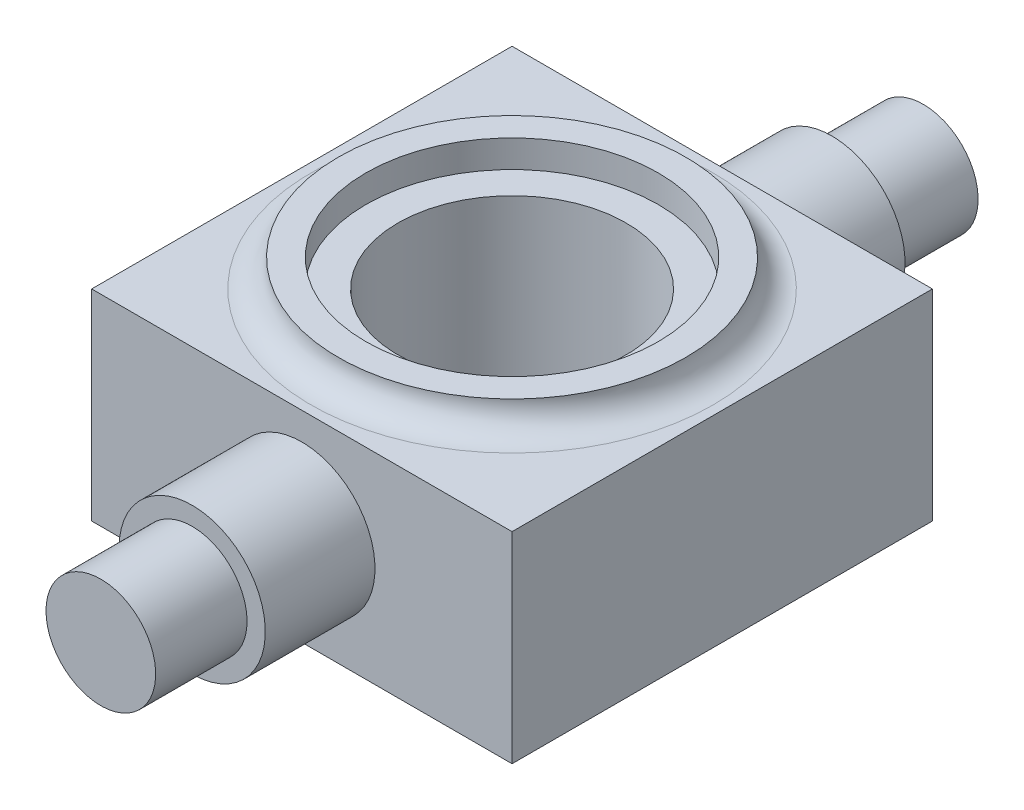
ISO-10303-21;
HEADER;
FILE_DESCRIPTION(('STEP AP214'),'2;1');
FILE_NAME('part.step','',(''),(''),'','','');
FILE_SCHEMA(('AUTOMOTIVE_DESIGN { 1 0 10303 214 1 1 1 1 }'));
ENDSEC;
DATA;
#1=APPLICATION_CONTEXT('core data for automotive mechanical design processes');
#2=APPLICATION_PROTOCOL_DEFINITION('international standard','automotive_design',2000,#1);
#3=PRODUCT_CONTEXT('',#1,'mechanical');
#4=PRODUCT('Part','Part','',(#3));
#5=PRODUCT_RELATED_PRODUCT_CATEGORY('part','',(#4));
#6=PRODUCT_DEFINITION_FORMATION('','',#4);
#7=PRODUCT_DEFINITION_CONTEXT('part definition',#1,'design');
#8=PRODUCT_DEFINITION('design','',#6,#7);
#9=PRODUCT_DEFINITION_SHAPE('','',#8);
#10=(LENGTH_UNIT() NAMED_UNIT(*) SI_UNIT(.MILLI.,.METRE.));
#11=(NAMED_UNIT(*) PLANE_ANGLE_UNIT() SI_UNIT($,.RADIAN.));
#12=(NAMED_UNIT(*) SI_UNIT($,.STERADIAN.) SOLID_ANGLE_UNIT());
#13=UNCERTAINTY_MEASURE_WITH_UNIT(LENGTH_MEASURE(1.E-05),#10,'distance_accuracy_value','');
#14=(GEOMETRIC_REPRESENTATION_CONTEXT(3) GLOBAL_UNCERTAINTY_ASSIGNED_CONTEXT((#13)) GLOBAL_UNIT_ASSIGNED_CONTEXT((#10,
#11,#12)) REPRESENTATION_CONTEXT('',''));
#15=CARTESIAN_POINT('',(0.,0.,0.));
#16=DIRECTION('',(0.,0.,1.));
#17=DIRECTION('',(1.,0.,0.));
#18=AXIS2_PLACEMENT_3D('',#15,#16,#17);
#19=CARTESIAN_POINT('',(-23.,-11.,23.));
#20=DIRECTION('',(1.,0.,0.));
#21=DIRECTION('',(0.,0.,-1.));
#22=AXIS2_PLACEMENT_3D('',#19,#20,#21);
#23=PLANE('',#22);
#24=DIRECTION('',(0.,-1.,0.));
#25=VECTOR('',#24,1.);
#26=CARTESIAN_POINT('',(-23.,-11.,-23.));
#27=LINE('',#26,#25);
#28=CARTESIAN_POINT('',(-23.,11.,-23.));
#29=VERTEX_POINT('',#28);
#30=CARTESIAN_POINT('',(-23.,-11.,-23.));
#31=VERTEX_POINT('',#30);
#32=EDGE_CURVE('E113',#29,#31,#27,.T.);
#33=ORIENTED_EDGE('',*,*,#32,.T.);
#34=DIRECTION('',(0.,0.,-1.));
#35=VECTOR('',#34,1.);
#36=CARTESIAN_POINT('',(-23.,-11.,23.));
#37=LINE('',#36,#35);
#38=CARTESIAN_POINT('',(-23.,-11.,23.));
#39=VERTEX_POINT('',#38);
#40=EDGE_CURVE('E104',#39,#31,#37,.T.);
#41=ORIENTED_EDGE('',*,*,#40,.F.);
#42=DIRECTION('',(0.,-1.,0.));
#43=VECTOR('',#42,1.);
#44=CARTESIAN_POINT('',(-23.,-11.,23.));
#45=LINE('',#44,#43);
#46=CARTESIAN_POINT('',(-23.,11.,23.));
#47=VERTEX_POINT('',#46);
#48=EDGE_CURVE('E96',#47,#39,#45,.T.);
#49=ORIENTED_EDGE('',*,*,#48,.F.);
#50=DIRECTION('',(0.,0.,-1.));
#51=VECTOR('',#50,1.);
#52=CARTESIAN_POINT('',(-23.,11.,23.));
#53=LINE('',#52,#51);
#54=EDGE_CURVE('E107',#47,#29,#53,.T.);
#55=ORIENTED_EDGE('',*,*,#54,.T.);
#56=EDGE_LOOP('',(#33,#41,#49,#55));
#57=FACE_BOUND('',#56,.T.);
#58=ADVANCED_FACE('F44',(#57),#23,.F.);
#59=CARTESIAN_POINT('',(23.,-11.,23.));
#60=DIRECTION('',(0.,1.,0.));
#61=DIRECTION('',(-1.,0.,0.));
#62=AXIS2_PLACEMENT_3D('',#59,#60,#61);
#63=PLANE('',#62);
#64=CARTESIAN_POINT('',(0.,-11.,0.));
#65=DIRECTION('',(0.,1.,0.));
#66=DIRECTION('',(-1.,0.,0.));
#67=AXIS2_PLACEMENT_3D('',#64,#65,#66);
#68=CIRCLE('',#67,22.);
#69=CARTESIAN_POINT('',(-22.,-11.,0.));
#70=VERTEX_POINT('',#69);
#71=EDGE_CURVE('E11',#70,#70,#68,.T.);
#72=ORIENTED_EDGE('',*,*,#71,.T.);
#73=EDGE_LOOP('',(#72));
#74=FACE_BOUND('',#73,.T.);
#75=DIRECTION('',(1.,0.,0.));
#76=VECTOR('',#75,1.);
#77=CARTESIAN_POINT('',(23.,-11.,-23.));
#78=LINE('',#77,#76);
#79=CARTESIAN_POINT('',(23.,-11.,-23.));
#80=VERTEX_POINT('',#79);
#81=EDGE_CURVE('E101',#31,#80,#78,.T.);
#82=ORIENTED_EDGE('',*,*,#81,.T.);
#83=DIRECTION('',(0.,0.,-1.));
#84=VECTOR('',#83,1.);
#85=CARTESIAN_POINT('',(23.,-11.,23.));
#86=LINE('',#85,#84);
#87=CARTESIAN_POINT('',(23.,-11.,23.));
#88=VERTEX_POINT('',#87);
#89=EDGE_CURVE('E103',#88,#80,#86,.T.);
#90=ORIENTED_EDGE('',*,*,#89,.F.);
#91=DIRECTION('',(1.,0.,0.));
#92=VECTOR('',#91,1.);
#93=CARTESIAN_POINT('',(23.,-11.,23.));
#94=LINE('',#93,#92);
#95=EDGE_CURVE('E95',#39,#88,#94,.T.);
#96=ORIENTED_EDGE('',*,*,#95,.F.);
#97=ORIENTED_EDGE('',*,*,#40,.T.);
#98=EDGE_LOOP('',(#82,#90,#96,#97));
#99=FACE_BOUND('',#98,.T.);
#100=ADVANCED_FACE('F105',(#74,#99),#63,.F.);
#101=CARTESIAN_POINT('',(23.,-11.,23.));
#102=DIRECTION('',(-1.,0.,0.));
#103=DIRECTION('',(0.,0.,1.));
#104=AXIS2_PLACEMENT_3D('',#101,#102,#103);
#105=PLANE('',#104);
#106=DIRECTION('',(0.,1.,0.));
#107=VECTOR('',#106,1.);
#108=CARTESIAN_POINT('',(23.,-11.,-23.));
#109=LINE('',#108,#107);
#110=CARTESIAN_POINT('',(23.,11.,-23.));
#111=VERTEX_POINT('',#110);
#112=EDGE_CURVE('E79',#80,#111,#109,.T.);
#113=ORIENTED_EDGE('',*,*,#112,.T.);
#114=DIRECTION('',(0.,0.,-1.));
#115=VECTOR('',#114,1.);
#116=CARTESIAN_POINT('',(23.,11.,23.));
#117=LINE('',#116,#115);
#118=CARTESIAN_POINT('',(23.,11.,23.));
#119=VERTEX_POINT('',#118);
#120=EDGE_CURVE('E102',#119,#111,#117,.T.);
#121=ORIENTED_EDGE('',*,*,#120,.F.);
#122=DIRECTION('',(0.,1.,0.));
#123=VECTOR('',#122,1.);
#124=CARTESIAN_POINT('',(23.,-11.,23.));
#125=LINE('',#124,#123);
#126=EDGE_CURVE('E98',#88,#119,#125,.T.);
#127=ORIENTED_EDGE('',*,*,#126,.F.);
#128=ORIENTED_EDGE('',*,*,#89,.T.);
#129=EDGE_LOOP('',(#113,#121,#127,#128));
#130=FACE_BOUND('',#129,.T.);
#131=ADVANCED_FACE('F110',(#130),#105,.F.);
#132=CARTESIAN_POINT('',(23.,11.,23.));
#133=DIRECTION('',(0.,-1.,0.));
#134=DIRECTION('',(1.,0.,0.));
#135=AXIS2_PLACEMENT_3D('',#132,#133,#134);
#136=PLANE('',#135);
#137=CARTESIAN_POINT('',(0.,11.,0.));
#138=DIRECTION('',(0.,-1.,0.));
#139=DIRECTION('',(1.,0.,0.));
#140=AXIS2_PLACEMENT_3D('',#137,#138,#139);
#141=CIRCLE('',#140,22.);
#142=CARTESIAN_POINT('',(22.,11.,0.));
#143=VERTEX_POINT('',#142);
#144=EDGE_CURVE('E53',#143,#143,#141,.T.);
#145=ORIENTED_EDGE('',*,*,#144,.T.);
#146=EDGE_LOOP('',(#145));
#147=FACE_BOUND('',#146,.T.);
#148=DIRECTION('',(-1.,0.,0.));
#149=VECTOR('',#148,1.);
#150=CARTESIAN_POINT('',(23.,11.,-23.));
#151=LINE('',#150,#149);
#152=EDGE_CURVE('E81',#111,#29,#151,.T.);
#153=ORIENTED_EDGE('',*,*,#152,.T.);
#154=ORIENTED_EDGE('',*,*,#54,.F.);
#155=DIRECTION('',(-1.,0.,0.));
#156=VECTOR('',#155,1.);
#157=CARTESIAN_POINT('',(23.,11.,23.));
#158=LINE('',#157,#156);
#159=EDGE_CURVE('E64',#119,#47,#158,.T.);
#160=ORIENTED_EDGE('',*,*,#159,.F.);
#161=ORIENTED_EDGE('',*,*,#120,.T.);
#162=EDGE_LOOP('',(#153,#154,#160,#161));
#163=FACE_BOUND('',#162,.T.);
#164=ADVANCED_FACE('F227',(#147,#163),#136,.F.);
#165=CARTESIAN_POINT('',(0.,0.,23.));
#166=DIRECTION('',(0.,0.,1.));
#167=DIRECTION('',(1.,0.,0.));
#168=AXIS2_PLACEMENT_3D('',#165,#166,#167);
#169=PLANE('',#168);
#170=CARTESIAN_POINT('',(0.,0.,23.));
#171=DIRECTION('',(0.,0.,-1.));
#172=DIRECTION('',(-1.,0.,0.));
#173=AXIS2_PLACEMENT_3D('',#170,#171,#172);
#174=CIRCLE('',#173,8.);
#175=CARTESIAN_POINT('',(-8.,0.,23.));
#176=VERTEX_POINT('',#175);
#177=EDGE_CURVE('E150',#176,#176,#174,.T.);
#178=ORIENTED_EDGE('',*,*,#177,.T.);
#179=EDGE_LOOP('',(#178));
#180=FACE_BOUND('',#179,.T.);
#181=ORIENTED_EDGE('',*,*,#48,.T.);
#182=ORIENTED_EDGE('',*,*,#95,.T.);
#183=ORIENTED_EDGE('',*,*,#126,.T.);
#184=ORIENTED_EDGE('',*,*,#159,.T.);
#185=EDGE_LOOP('',(#181,#182,#183,#184));
#186=FACE_BOUND('',#185,.T.);
#187=ADVANCED_FACE('F93',(#180,#186),#169,.T.);
#188=CARTESIAN_POINT('',(0.,0.,-23.));
#189=DIRECTION('',(0.,0.,1.));
#190=DIRECTION('',(1.,0.,0.));
#191=AXIS2_PLACEMENT_3D('',#188,#189,#190);
#192=PLANE('',#191);
#193=CARTESIAN_POINT('',(0.,0.,-23.));
#194=DIRECTION('',(0.,0.,-1.));
#195=DIRECTION('',(-1.,0.,0.));
#196=AXIS2_PLACEMENT_3D('',#193,#194,#195);
#197=CIRCLE('',#196,8.);
#198=CARTESIAN_POINT('',(-8.,0.,-23.));
#199=VERTEX_POINT('',#198);
#200=EDGE_CURVE('E124',#199,#199,#197,.T.);
#201=ORIENTED_EDGE('',*,*,#200,.F.);
#202=EDGE_LOOP('',(#201));
#203=FACE_BOUND('',#202,.T.);
#204=ORIENTED_EDGE('',*,*,#32,.F.);
#205=ORIENTED_EDGE('',*,*,#152,.F.);
#206=ORIENTED_EDGE('',*,*,#112,.F.);
#207=ORIENTED_EDGE('',*,*,#81,.F.);
#208=EDGE_LOOP('',(#204,#205,#206,#207));
#209=FACE_BOUND('',#208,.T.);
#210=ADVANCED_FACE('F230',(#203,#209),#192,.F.);
#211=CARTESIAN_POINT('',(0.,0.,-35.));
#212=DIRECTION('',(0.,0.,1.));
#213=DIRECTION('',(1.,0.,0.));
#214=AXIS2_PLACEMENT_3D('',#211,#212,#213);
#215=CYLINDRICAL_SURFACE('',#214,8.);
#216=CARTESIAN_POINT('',(0.,0.,-35.));
#217=DIRECTION('',(0.,0.,-1.));
#218=DIRECTION('',(-1.,0.,0.));
#219=AXIS2_PLACEMENT_3D('',#216,#217,#218);
#220=CIRCLE('',#219,8.);
#221=CARTESIAN_POINT('',(-8.,0.,-35.));
#222=VERTEX_POINT('',#221);
#223=EDGE_CURVE('E116',#222,#222,#220,.T.);
#224=ORIENTED_EDGE('',*,*,#223,.F.);
#225=EDGE_LOOP('',(#224));
#226=FACE_BOUND('',#225,.T.);
#227=ORIENTED_EDGE('',*,*,#200,.T.);
#228=EDGE_LOOP('',(#227));
#229=FACE_BOUND('',#228,.T.);
#230=ADVANCED_FACE('F235',(#226,#229),#215,.T.);
#231=CARTESIAN_POINT('',(0.,0.,-35.));
#232=DIRECTION('',(0.,0.,-1.));
#233=DIRECTION('',(-1.,0.,0.));
#234=AXIS2_PLACEMENT_3D('',#231,#232,#233);
#235=PLANE('',#234);
#236=CARTESIAN_POINT('',(0.,0.,-35.));
#237=DIRECTION('',(0.,0.,-1.));
#238=DIRECTION('',(-1.,0.,0.));
#239=AXIS2_PLACEMENT_3D('',#236,#237,#238);
#240=CIRCLE('',#239,6.);
#241=CARTESIAN_POINT('',(-6.,0.,-35.));
#242=VERTEX_POINT('',#241);
#243=EDGE_CURVE('E127',#242,#242,#240,.T.);
#244=ORIENTED_EDGE('',*,*,#243,.F.);
#245=EDGE_LOOP('',(#244));
#246=FACE_BOUND('',#245,.T.);
#247=ORIENTED_EDGE('',*,*,#223,.T.);
#248=EDGE_LOOP('',(#247));
#249=FACE_BOUND('',#248,.T.);
#250=ADVANCED_FACE('F237',(#246,#249),#235,.T.);
#251=CARTESIAN_POINT('',(0.,0.,-45.));
#252=DIRECTION('',(0.,0.,1.));
#253=DIRECTION('',(1.,0.,0.));
#254=AXIS2_PLACEMENT_3D('',#251,#252,#253);
#255=CYLINDRICAL_SURFACE('',#254,6.);
#256=CARTESIAN_POINT('',(0.,0.,-45.));
#257=DIRECTION('',(0.,0.,-1.));
#258=DIRECTION('',(-1.,0.,0.));
#259=AXIS2_PLACEMENT_3D('',#256,#257,#258);
#260=CIRCLE('',#259,6.);
#261=CARTESIAN_POINT('',(-6.,0.,-45.));
#262=VERTEX_POINT('',#261);
#263=EDGE_CURVE('E138',#262,#262,#260,.T.);
#264=ORIENTED_EDGE('',*,*,#263,.F.);
#265=EDGE_LOOP('',(#264));
#266=FACE_BOUND('',#265,.T.);
#267=ORIENTED_EDGE('',*,*,#243,.T.);
#268=EDGE_LOOP('',(#267));
#269=FACE_BOUND('',#268,.T.);
#270=ADVANCED_FACE('F243',(#266,#269),#255,.T.);
#271=CARTESIAN_POINT('',(0.,0.,-45.));
#272=DIRECTION('',(0.,0.,-1.));
#273=DIRECTION('',(-1.,0.,0.));
#274=AXIS2_PLACEMENT_3D('',#271,#272,#273);
#275=PLANE('',#274);
#276=ORIENTED_EDGE('',*,*,#263,.T.);
#277=EDGE_LOOP('',(#276));
#278=FACE_BOUND('',#277,.T.);
#279=ADVANCED_FACE('F250',(#278),#275,.T.);
#280=CARTESIAN_POINT('',(0.,0.,35.));
#281=DIRECTION('',(0.,0.,-1.));
#282=DIRECTION('',(-1.,0.,0.));
#283=AXIS2_PLACEMENT_3D('',#280,#281,#282);
#284=CYLINDRICAL_SURFACE('',#283,8.);
#285=CARTESIAN_POINT('',(0.,0.,35.));
#286=DIRECTION('',(0.,0.,-1.));
#287=DIRECTION('',(-1.,0.,0.));
#288=AXIS2_PLACEMENT_3D('',#285,#286,#287);
#289=CIRCLE('',#288,8.);
#290=CARTESIAN_POINT('',(-8.,0.,35.));
#291=VERTEX_POINT('',#290);
#292=EDGE_CURVE('E143',#291,#291,#289,.T.);
#293=ORIENTED_EDGE('',*,*,#292,.T.);
#294=EDGE_LOOP('',(#293));
#295=FACE_BOUND('',#294,.T.);
#296=ORIENTED_EDGE('',*,*,#177,.F.);
#297=EDGE_LOOP('',(#296));
#298=FACE_BOUND('',#297,.T.);
#299=ADVANCED_FACE('F252',(#295,#298),#284,.T.);
#300=CARTESIAN_POINT('',(0.,0.,35.));
#301=DIRECTION('',(0.,0.,1.));
#302=DIRECTION('',(-1.,0.,0.));
#303=AXIS2_PLACEMENT_3D('',#300,#301,#302);
#304=PLANE('',#303);
#305=CARTESIAN_POINT('',(0.,0.,35.));
#306=DIRECTION('',(0.,0.,-1.));
#307=DIRECTION('',(-1.,0.,0.));
#308=AXIS2_PLACEMENT_3D('',#305,#306,#307);
#309=CIRCLE('',#308,6.);
#310=CARTESIAN_POINT('',(-6.,0.,35.));
#311=VERTEX_POINT('',#310);
#312=EDGE_CURVE('E159',#311,#311,#309,.T.);
#313=ORIENTED_EDGE('',*,*,#312,.T.);
#314=EDGE_LOOP('',(#313));
#315=FACE_BOUND('',#314,.T.);
#316=ORIENTED_EDGE('',*,*,#292,.F.);
#317=EDGE_LOOP('',(#316));
#318=FACE_BOUND('',#317,.T.);
#319=ADVANCED_FACE('F251',(#315,#318),#304,.T.);
#320=CARTESIAN_POINT('',(0.,0.,45.));
#321=DIRECTION('',(0.,0.,-1.));
#322=DIRECTION('',(-1.,0.,0.));
#323=AXIS2_PLACEMENT_3D('',#320,#321,#322);
#324=CYLINDRICAL_SURFACE('',#323,6.);
#325=CARTESIAN_POINT('',(0.,0.,45.));
#326=DIRECTION('',(0.,0.,-1.));
#327=DIRECTION('',(-1.,0.,0.));
#328=AXIS2_PLACEMENT_3D('',#325,#326,#327);
#329=CIRCLE('',#328,6.);
#330=CARTESIAN_POINT('',(-6.,0.,45.));
#331=VERTEX_POINT('',#330);
#332=EDGE_CURVE('E154',#331,#331,#329,.T.);
#333=ORIENTED_EDGE('',*,*,#332,.T.);
#334=EDGE_LOOP('',(#333));
#335=FACE_BOUND('',#334,.T.);
#336=ORIENTED_EDGE('',*,*,#312,.F.);
#337=EDGE_LOOP('',(#336));
#338=FACE_BOUND('',#337,.T.);
#339=ADVANCED_FACE('F259',(#335,#338),#324,.T.);
#340=CARTESIAN_POINT('',(0.,0.,45.));
#341=DIRECTION('',(0.,0.,1.));
#342=DIRECTION('',(-1.,0.,0.));
#343=AXIS2_PLACEMENT_3D('',#340,#341,#342);
#344=PLANE('',#343);
#345=ORIENTED_EDGE('',*,*,#332,.F.);
#346=EDGE_LOOP('',(#345));
#347=FACE_BOUND('',#346,.T.);
#348=ADVANCED_FACE('F204',(#347),#344,.T.);
#349=CARTESIAN_POINT('',(0.,14.,0.));
#350=DIRECTION('',(0.,1.,0.));
#351=DIRECTION('',(-1.,0.,0.));
#352=AXIS2_PLACEMENT_3D('',#349,#350,#351);
#353=PLANE('',#352);
#354=CARTESIAN_POINT('',(0.,14.,0.));
#355=DIRECTION('',(0.,1.,0.));
#356=DIRECTION('',(-1.,0.,0.));
#357=AXIS2_PLACEMENT_3D('',#354,#355,#356);
#358=CIRCLE('',#357,16.);
#359=CARTESIAN_POINT('',(-16.,14.,0.));
#360=VERTEX_POINT('',#359);
#361=EDGE_CURVE('E164',#360,#360,#358,.T.);
#362=ORIENTED_EDGE('',*,*,#361,.F.);
#363=EDGE_LOOP('',(#362));
#364=FACE_BOUND('',#363,.T.);
#365=CARTESIAN_POINT('',(0.,14.,0.));
#366=DIRECTION('',(0.,1.,0.));
#367=DIRECTION('',(-1.,0.,0.));
#368=AXIS2_PLACEMENT_3D('',#365,#366,#367);
#369=CIRCLE('',#368,19.);
#370=CARTESIAN_POINT('',(-19.,14.,0.));
#371=VERTEX_POINT('',#370);
#372=EDGE_CURVE('E158',#371,#371,#369,.T.);
#373=ORIENTED_EDGE('',*,*,#372,.T.);
#374=EDGE_LOOP('',(#373));
#375=FACE_BOUND('',#374,.T.);
#376=ADVANCED_FACE('F191',(#364,#375),#353,.T.);
#377=CARTESIAN_POINT('',(0.,11.,0.));
#378=DIRECTION('',(0.,1.,0.));
#379=DIRECTION('',(-1.,0.,0.));
#380=AXIS2_PLACEMENT_3D('',#377,#378,#379);
#381=CYLINDRICAL_SURFACE('',#380,16.);
#382=CARTESIAN_POINT('',(0.,11.,0.));
#383=DIRECTION('',(0.,1.,0.));
#384=DIRECTION('',(-1.,0.,0.));
#385=AXIS2_PLACEMENT_3D('',#382,#383,#384);
#386=CIRCLE('',#385,16.);
#387=CARTESIAN_POINT('',(-16.,11.,0.));
#388=VERTEX_POINT('',#387);
#389=EDGE_CURVE('E165',#388,#388,#386,.T.);
#390=ORIENTED_EDGE('',*,*,#389,.F.);
#391=EDGE_LOOP('',(#390));
#392=FACE_BOUND('',#391,.T.);
#393=ORIENTED_EDGE('',*,*,#361,.T.);
#394=EDGE_LOOP('',(#393));
#395=FACE_BOUND('',#394,.T.);
#396=ADVANCED_FACE('F186',(#392,#395),#381,.F.);
#397=CARTESIAN_POINT('',(0.,11.,0.));
#398=DIRECTION('',(0.,1.,0.));
#399=DIRECTION('',(-1.,0.,0.));
#400=AXIS2_PLACEMENT_3D('',#397,#398,#399);
#401=PLANE('',#400);
#402=CARTESIAN_POINT('',(0.,11.,0.));
#403=DIRECTION('',(0.,1.,0.));
#404=DIRECTION('',(-1.,0.,0.));
#405=AXIS2_PLACEMENT_3D('',#402,#403,#404);
#406=CIRCLE('',#405,12.5);
#407=CARTESIAN_POINT('',(-12.5,11.,0.));
#408=VERTEX_POINT('',#407);
#409=EDGE_CURVE('E128',#408,#408,#406,.T.);
#410=ORIENTED_EDGE('',*,*,#409,.F.);
#411=EDGE_LOOP('',(#410));
#412=FACE_BOUND('',#411,.T.);
#413=ORIENTED_EDGE('',*,*,#389,.T.);
#414=EDGE_LOOP('',(#413));
#415=FACE_BOUND('',#414,.T.);
#416=ADVANCED_FACE('F184',(#412,#415),#401,.T.);
#417=CARTESIAN_POINT('',(0.,-14.,0.));
#418=DIRECTION('',(0.,-1.,0.));
#419=DIRECTION('',(-1.,0.,0.));
#420=AXIS2_PLACEMENT_3D('',#417,#418,#419);
#421=PLANE('',#420);
#422=CARTESIAN_POINT('',(0.,-14.,0.));
#423=DIRECTION('',(0.,1.,0.));
#424=DIRECTION('',(-1.,0.,0.));
#425=AXIS2_PLACEMENT_3D('',#422,#423,#424);
#426=CIRCLE('',#425,16.);
#427=CARTESIAN_POINT('',(-16.,-14.,0.));
#428=VERTEX_POINT('',#427);
#429=EDGE_CURVE('E172',#428,#428,#426,.T.);
#430=ORIENTED_EDGE('',*,*,#429,.T.);
#431=EDGE_LOOP('',(#430));
#432=FACE_BOUND('',#431,.T.);
#433=CARTESIAN_POINT('',(0.,-14.,0.));
#434=DIRECTION('',(0.,1.,0.));
#435=DIRECTION('',(-1.,0.,0.));
#436=AXIS2_PLACEMENT_3D('',#433,#434,#435);
#437=CIRCLE('',#436,19.);
#438=CARTESIAN_POINT('',(-19.,-14.,0.));
#439=VERTEX_POINT('',#438);
#440=EDGE_CURVE('E166',#439,#439,#437,.T.);
#441=ORIENTED_EDGE('',*,*,#440,.F.);
#442=EDGE_LOOP('',(#441));
#443=FACE_BOUND('',#442,.T.);
#444=ADVANCED_FACE('F189',(#432,#443),#421,.T.);
#445=CARTESIAN_POINT('',(0.,-11.,0.));
#446=DIRECTION('',(0.,-1.,0.));
#447=DIRECTION('',(1.,0.,0.));
#448=AXIS2_PLACEMENT_3D('',#445,#446,#447);
#449=CYLINDRICAL_SURFACE('',#448,16.);
#450=CARTESIAN_POINT('',(0.,-11.,0.));
#451=DIRECTION('',(0.,1.,0.));
#452=DIRECTION('',(-1.,0.,0.));
#453=AXIS2_PLACEMENT_3D('',#450,#451,#452);
#454=CIRCLE('',#453,16.);
#455=CARTESIAN_POINT('',(-16.,-11.,0.));
#456=VERTEX_POINT('',#455);
#457=EDGE_CURVE('E173',#456,#456,#454,.T.);
#458=ORIENTED_EDGE('',*,*,#457,.T.);
#459=EDGE_LOOP('',(#458));
#460=FACE_BOUND('',#459,.T.);
#461=ORIENTED_EDGE('',*,*,#429,.F.);
#462=EDGE_LOOP('',(#461));
#463=FACE_BOUND('',#462,.T.);
#464=ADVANCED_FACE('F266',(#460,#463),#449,.F.);
#465=CARTESIAN_POINT('',(0.,-11.,0.));
#466=DIRECTION('',(0.,-1.,0.));
#467=DIRECTION('',(-1.,0.,0.));
#468=AXIS2_PLACEMENT_3D('',#465,#466,#467);
#469=PLANE('',#468);
#470=CARTESIAN_POINT('',(0.,-11.,0.));
#471=DIRECTION('',(0.,-1.,0.));
#472=DIRECTION('',(1.,0.,0.));
#473=AXIS2_PLACEMENT_3D('',#470,#471,#472);
#474=CIRCLE('',#473,12.5);
#475=CARTESIAN_POINT('',(12.5,-11.,0.));
#476=VERTEX_POINT('',#475);
#477=EDGE_CURVE('E121',#476,#476,#474,.T.);
#478=ORIENTED_EDGE('',*,*,#477,.F.);
#479=EDGE_LOOP('',(#478));
#480=FACE_BOUND('',#479,.T.);
#481=ORIENTED_EDGE('',*,*,#457,.F.);
#482=EDGE_LOOP('',(#481));
#483=FACE_BOUND('',#482,.T.);
#484=ADVANCED_FACE('F215',(#480,#483),#469,.T.);
#485=CARTESIAN_POINT('',(0.,-14.,0.));
#486=DIRECTION('',(0.,1.,0.));
#487=DIRECTION('',(-1.,0.,0.));
#488=AXIS2_PLACEMENT_3D('',#485,#486,#487);
#489=CYLINDRICAL_SURFACE('',#488,12.5);
#490=ORIENTED_EDGE('',*,*,#409,.T.);
#491=EDGE_LOOP('',(#490));
#492=FACE_BOUND('',#491,.T.);
#493=ORIENTED_EDGE('',*,*,#477,.T.);
#494=EDGE_LOOP('',(#493));
#495=FACE_BOUND('',#494,.T.);
#496=ADVANCED_FACE('F185',(#492,#495),#489,.F.);
#497=CARTESIAN_POINT('',(0.,14.,0.));
#498=DIRECTION('',(0.,-1.,0.));
#499=DIRECTION('',(1.,0.,0.));
#500=AXIS2_PLACEMENT_3D('',#497,#498,#499);
#501=TOROIDAL_SURFACE('',#500,22.,3.);
#502=ORIENTED_EDGE('',*,*,#144,.F.);
#503=EDGE_LOOP('',(#502));
#504=FACE_BOUND('',#503,.T.);
#505=ORIENTED_EDGE('',*,*,#372,.F.);
#506=EDGE_LOOP('',(#505));
#507=FACE_BOUND('',#506,.T.);
#508=ADVANCED_FACE('F202',(#504,#507),#501,.F.);
#509=CARTESIAN_POINT('',(0.,-14.,0.));
#510=DIRECTION('',(0.,1.,0.));
#511=DIRECTION('',(-1.,0.,0.));
#512=AXIS2_PLACEMENT_3D('',#509,#510,#511);
#513=TOROIDAL_SURFACE('',#512,22.,3.);
#514=ORIENTED_EDGE('',*,*,#440,.T.);
#515=EDGE_LOOP('',(#514));
#516=FACE_BOUND('',#515,.T.);
#517=ORIENTED_EDGE('',*,*,#71,.F.);
#518=EDGE_LOOP('',(#517));
#519=FACE_BOUND('',#518,.T.);
#520=ADVANCED_FACE('F50',(#516,#519),#513,.F.);
#521=CLOSED_SHELL('',(#58,#100,#131,#164,#187,#210,#230,#250,#270,#279,#299,#319,#339,#348,#376,
#396,#416,#444,#464,#484,#496,#508,#520));
#522=MANIFOLD_SOLID_BREP('B2',#521);
#523=ADVANCED_BREP_SHAPE_REPRESENTATION('',(#18,#522),#14);
#524=SHAPE_DEFINITION_REPRESENTATION(#9,#523);
ENDSEC;
END-ISO-10303-21;
